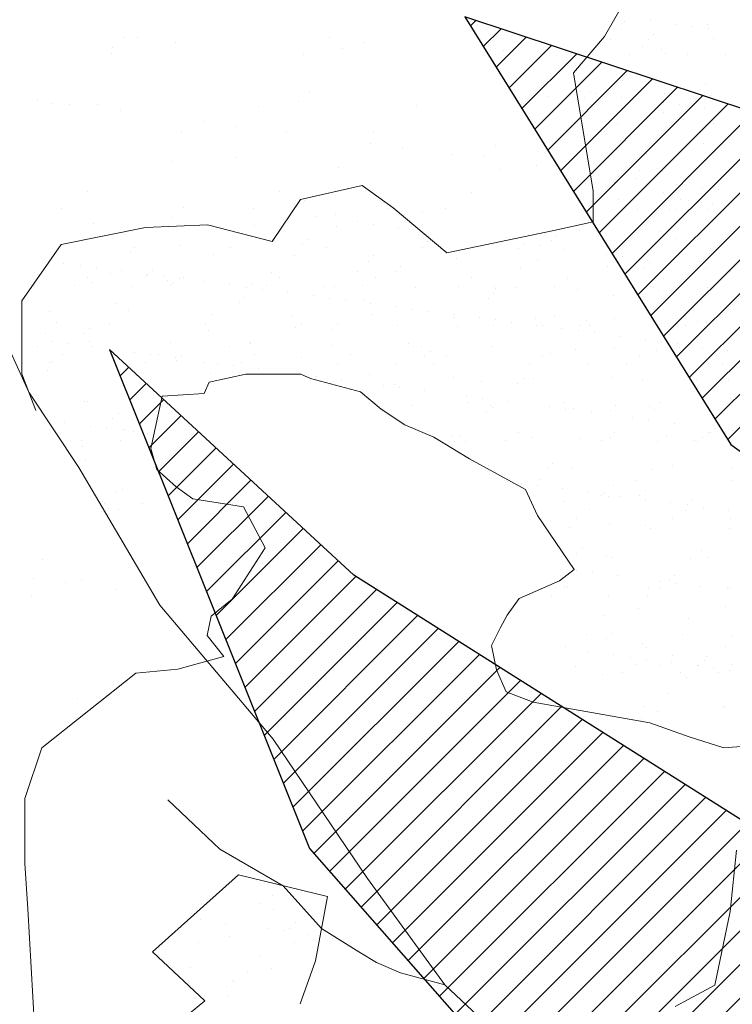
# Model space of a CAD drawing. Units: inches. Extents: x 1986 to 21484, y -1816 to 2016.
# Tile 22 of 85: x 2157.681 to 2162.297, y 1891.95 to 1898.331. Entities that reach past the tile are written whole.
import ezdxf

# ---------------------------------------------------------------- set-up
doc = ezdxf.new("R2010")
doc.units = ezdxf.units.IN
doc.layers.add('L-PLNT', color=84, linetype='Continuous', lineweight=13)
doc.layers.add('vfolhas', color=114, linetype='Continuous', lineweight=5)
doc.layers.add('vfolha2', color=110, linetype='Continuous')
doc.layers.add('vfolhas2', color=102, linetype='Continuous')
pattern_1 = [(45, (-2446.5133113, 50.986076), (-0.004419417382, 0.004419417382), [])]

# ---------------------------------------------------------------- blocks, each defined once
blk = doc.blocks.new('arbusto_PB_verde_grande')
at = {"layer": 'vfolha2'}
h = blk.add_hatch(dxfattribs=at)
h.set_pattern_fill('ANSI31', color=256, scale=0.05, style=0)
h.set_pattern_definition(pattern_1)
h.paths.add_polyline_path([(-0.18963, 0.29704), (-0.08553, 0.20192), (-0.10785, 0.25007), (-0.13202, 0.31865), (-0.25096, 0.48479), (-0.44952, 0.5505), (-0.37946, 0.43789)])
h.paths.add_polyline_path([(0.07911, -0.4071), (0.08214, -0.50631), (0.17255, -0.6355), (0.18428, -0.44151), (0.14904, -0.29177), (0.02625, -0.03934), (0.03527, -0.25376)])
at = {"layer": 'vfolhas'}
h = blk.add_hatch(dxfattribs=at)
h.set_pattern_fill('ANSI31', color=256, scale=0.05, style=0)
h.set_pattern_definition(pattern_1)
h.paths.add_polyline_path([(-0.07279, 0.50669), (-0.18085, 0.65063), (-0.2334, 0.67253), (-0.20712, 0.53176), (-0.10785, 0.25007), (0.02625, -0.03934), (0.00028, 0.09048), (0.00816, 0.16241), (-0.04939, 0.29079)])
h.paths.add_polyline_path([(0.09902, 0.41929), (0.09372, 0.26573), (0.07906, 0.18814), (0.15506, 0.36901), (0.26606, 0.5505), (0.28356, 0.63504), (0.2485, 0.68819), (0.25145, 0.63504), (0.20178, 0.54426)])
h.paths.add_polyline_path([(0.12295, 0.24073), (0.047, 0.06233), (0.02625, -0.03934), (0.11122, 0.04358), (0.18428, 0.09364), (0.27478, 0.19376), (0.3215, 0.25323), (0.44129, 0.38467), (0.47634, 0.57866), (0.41789, 0.45347), (0.28939, 0.30954)])
h.paths.add_polyline_path([(0.58145, -0.03779), (0.70707, 0.01536), (0.78591, 0.04667), (0.74796, 0.06549), (0.62818, 0.08423), (0.52595, 0.09048), (0.39745, 0.04358), (0.02625, -0.03934), (0.25728, -0.03154), (0.43834, -0.0347)])
h.paths.add_polyline_path([(0.52022, -0.03647), (0.43834, -0.0347), (0.25728, -0.03154), (0.02625, -0.03934), (0.17964, -0.08515), (0.53768, -0.13167), (0.69541, -0.15357), (0.78591, -0.07852), (0.70413, -0.10042)])
h.paths.add_polyline_path([(0.27189, -0.21929), (0.14922, -0.14107), (0.02625, -0.03934), (0.15794, -0.31007), (0.29522, -0.42585), (0.41789, -0.49157), (0.56396, -0.56669), (0.5114, -0.48532), (0.39456, -0.34139)])
h.paths.add_polyline_path([(-0.05818, -0.47591), (-0.02312, -0.61984), (0.047, -0.80134), (0.08494, -0.59794), (0.07911, -0.4071), (0.03527, -0.25376), (0.02625, -0.03934), (-0.03773, -0.26001)])
h.paths.add_polyline_path([(-0.24218, 0.14054), (-0.11073, 0.06858), (0.02625, -0.03934), (-0.04235, 0.10871), (-0.21007, 0.23757), (-0.36485, 0.33145), (-0.47874, 0.40341), (-0.54303, 0.46288), (-0.49041, 0.33145), (-0.39408, 0.22192)])
at = {"layer": 'vfolha2'}
for p, q in [((-0.44952, 0.5505), (-0.37946, 0.43789)), ((-0.25096, 0.48479), (-0.44952, 0.5505)), ((-0.37946, 0.43789), (-0.18963, 0.29704))]:
    blk.add_line(p, q, dxfattribs=at)
at = {"layer": 'vfolhas2'}
for p, q in [((-0.54303, 0.46288), (-0.49041, 0.33145)), ((-0.47874, 0.40341), (-0.54303, 0.46288)), ((-0.36485, 0.33145), (-0.47874, 0.40341)), ((-0.49041, 0.33145), (-0.39408, 0.22192))]:
    blk.add_line(p, q, dxfattribs=at)
blk = doc.blocks.new('PLANT-SHRUB')
for p, q in [((2161.4678, 1898.2224), (2161.6137, 1898.4774)), ((2161.5972, 1898.3209), (2161.5972, 1898.3209)), ((2161.7646, 1898.3226), (2161.7646, 1898.3226)), ((2161.9271, 1898.3012), (2161.9271, 1898.3012)), ((2161.9271, 1898.3012), (2161.9271, 1898.3012)), ((2162.0361, 1898.2868), (2162.0361, 1898.2868)), ((2162.1369, 1898.3014), (2162.1369, 1898.3014)), ((2161.2673, 1897.9855), (2161.4678, 1898.2224)), ((2161.5796, 1898.2672), (2161.5796, 1898.2672)), ((2161.5796, 1898.2672), (2161.5796, 1898.2672)), ((2161.7885, 1898.2334), (2161.7885, 1898.2334)), ((2162.1401, 1898.2731), (2162.1401, 1898.2731)), ((2158.3575, 1898.2181), (2158.3575, 1898.2181)), ((2158.4425, 1898.2174), (2158.4425, 1898.2174)), ((2158.6902, 1898.1833), (2158.6902, 1898.1833)), ((2159.6871, 1898.2151), (2159.6871, 1898.2151)), ((2159.9066, 1898.186), (2159.9066, 1898.186)), ((2160.9317, 1898.2128), (2160.9317, 1898.2128)), ((2161.5059, 1898.1997), (2161.5059, 1898.1997)), ((2161.5059, 1898.1997), (2161.5059, 1898.1997)), ((2161.7156, 1898.158), (2161.7156, 1898.158)), ((2161.7517, 1898.1997), (2161.7517, 1898.1997)), ((2162.1764, 1898.2106), (2162.1764, 1898.2106)), ((2162.1764, 1898.2106), (2162.1764, 1898.2106)), ((2158.2739, 1898.11), (2158.2739, 1898.11)), ((2158.2838, 1898.1506), (2158.2838, 1898.1506)), ((2159.5186, 1898.1077), (2159.5186, 1898.1077)), ((2159.7696, 1898.1444), (2159.7696, 1898.1444)), ((2160.7632, 1898.1055), (2160.7632, 1898.1055)), ((2160.8158, 1898.1311), (2160.8158, 1898.1311)), ((2161.6313, 1898.1043), (2161.6313, 1898.1043)), ((2161.8382, 1898.136), (2161.8382, 1898.136)), ((2161.8382, 1898.136), (2161.8382, 1898.136)), ((2161.8667, 1898.1141), (2161.8667, 1898.1141)), ((2162.0078, 1898.1032), (2162.0078, 1898.1032)), ((2162.0078, 1898.1032), (2162.0078, 1898.1032)), ((2162.2536, 1898.1032), (2162.2536, 1898.1032)), ((2161.3949, 1897.2203), (2161.2673, 1897.9855)), ((2161.5528, 1898.0174), (2161.5528, 1898.0174)), ((2161.5846, 1897.9358), (2161.5846, 1897.9358)), ((2162.1244, 1897.9164), (2162.1244, 1897.9164)), ((2159.5589, 1897.8673), (2159.5589, 1897.8673)), ((2161.3139, 1897.8645), (2161.3139, 1897.8645)), ((2161.379, 1897.8581), (2161.379, 1897.8581)), ((2161.4179, 1897.8508), (2161.4179, 1897.8508)), ((2161.8576, 1897.8509), (2161.8576, 1897.8509)), ((2162.1535, 1897.842), (2162.1535, 1897.842)), ((2157.7982, 1897.81), (2157.7982, 1897.81)), ((2157.886, 1897.7861), (2157.886, 1897.7861)), ((2158.0062, 1897.7826), (2158.0062, 1897.7826)), ((2158.183, 1897.783), (2158.183, 1897.783)), ((2159.4853, 1897.7998), (2159.4853, 1897.7998)), ((2161.1081, 1897.8352), (2161.1081, 1897.8352)), ((2161.3421, 1897.8244), (2161.3421, 1897.8244)), ((2161.5804, 1897.8294), (2161.5804, 1897.8294)), ((2161.8518, 1897.7937), (2161.8518, 1897.7937)), ((2161.9558, 1897.78), (2161.9558, 1897.78)), ((2158.3311, 1897.7398), (2158.3311, 1897.7398)), ((2159.2292, 1897.7697), (2159.2292, 1897.7697)), ((2160.2516, 1897.7746), (2160.2516, 1897.7746)), ((2161.3311, 1897.7357), (2161.3311, 1897.7357)), ((2161.3311, 1897.7357), (2161.3311, 1897.7357)), ((2161.3311, 1897.7357), (2161.3311, 1897.7357)), ((2161.8541, 1897.729), (2161.8541, 1897.729)), ((2162.1183, 1897.7586), (2162.1183, 1897.7586)), ((2158.874, 1897.6683), (2158.874, 1897.6683)), ((2161.5542, 1897.6576), (2161.5542, 1897.6576)), ((2161.9429, 1897.649), (2161.9429, 1897.649)), ((2161.9797, 1897.6827), (2161.9797, 1897.6827)), ((2162.1765, 1897.6565), (2162.1765, 1897.6565)), ((2158.7264, 1897.6031), (2158.7264, 1897.6031)), ((2159.082, 1897.6409), (2159.082, 1897.6409)), ((2159.4069, 1897.5982), (2159.4069, 1897.5982)), ((2159.9711, 1897.6008), (2159.9711, 1897.6008)), ((2161.2157, 1897.5986), (2161.2157, 1897.5986)), ((2161.4699, 1897.6039), (2161.4699, 1897.6039)), ((2162.0922, 1897.6028), (2162.0922, 1897.6028)), ((2159.9498, 1897.5267), (2159.9498, 1897.5267)), ((2161.572, 1897.5508), (2161.572, 1897.5508)), ((2162.1118, 1897.5313), (2162.1118, 1897.5313)), ((2160.1578, 1897.4993), (2160.1578, 1897.4993)), ((2160.4828, 1897.4565), (2160.4828, 1897.4565)), ((2160.7604, 1897.5166), (2160.7604, 1897.5166)), ((2161.7439, 1897.4667), (2161.7439, 1897.4667)), ((2158.665, 1897.4132), (2158.665, 1897.4132)), ((2159.0875, 1897.4353), (2159.0875, 1897.4353)), ((2160.6867, 1897.449), (2160.6867, 1897.449)), ((2159.7444, 1897.3743), (2159.7444, 1897.3743)), ((2160.7906, 1897.361), (2160.7906, 1897.361)), ((2161.0256, 1897.3851), (2161.0256, 1897.3851)), ((2161.2337, 1897.3577), (2161.2337, 1897.3577)), ((2161.3961, 1897.3363), (2161.3961, 1897.3363)), ((2161.6962, 1897.3505), (2161.6962, 1897.3505)), ((2161.813, 1897.3659), (2161.813, 1897.3659)), ((2161.813, 1897.3659), (2161.813, 1897.3659)), ((2161.8416, 1897.344), (2161.8416, 1897.344)), ((2161.5333, 1897.2737), (2161.5333, 1897.2737)), ((2161.5586, 1897.3149), (2161.5586, 1897.3149)), ((2161.5586, 1897.3149), (2161.5586, 1897.3149)), ((2161.5701, 1897.3074), (2161.5701, 1897.3074)), ((2161.6676, 1897.3005), (2161.6676, 1897.3005)), ((2161.7716, 1897.2869), (2161.7716, 1897.2869)), ((2161.934, 1897.2655), (2161.934, 1897.2655)), ((2158.1197, 1897.2165), (2158.1197, 1897.2165)), ((2159.3643, 1897.2143), (2159.3643, 1897.2143)), ((2159.4986, 1897.1656), (2159.8997, 1897.2567)), ((2159.8997, 1897.2567), (2160.1003, 1897.1109)), ((2159.8997, 1897.2567), (2159.8997, 1897.2567)), ((2160.6089, 1897.212), (2160.6089, 1897.212)), ((2161.3949, 1897.0199), (2161.3949, 1897.2203)), ((2161.8536, 1897.2098), (2161.8536, 1897.2098)), ((2161.8536, 1897.2098), (2161.8536, 1897.2098)), ((2162.1015, 1897.2434), (2162.1015, 1897.2434)), ((2162.1015, 1897.2434), (2162.1015, 1897.2434)), ((2162.2055, 1897.2297), (2162.2055, 1897.2297)), ((2159.3162, 1896.8923), (2159.4986, 1897.1656)), ((2159.5258, 1897.1606), (2159.5258, 1897.1606)), ((2159.9854, 1897.1894), (2159.9854, 1897.1894)), ((2161.5594, 1897.1657), (2161.5594, 1897.1657)), ((2161.9619, 1897.1658), (2161.9619, 1897.1658)), ((2161.9619, 1897.1658), (2161.9619, 1897.1658)), ((2162.0151, 1897.1561), (2162.0151, 1897.1561)), ((2162.0992, 1897.1463), (2162.0992, 1897.1463)), ((2157.9511, 1897.1092), (2157.9511, 1897.1092)), ((2158.7398, 1897.1167), (2158.7398, 1897.1167)), ((2159.1958, 1897.1069), (2159.1958, 1897.1069)), ((2160.0639, 1897.1058), (2160.0639, 1897.1058)), ((2160.1003, 1897.1109), (2160.4467, 1896.8194)), ((2160.2889, 1897.0845), (2160.2889, 1897.0845)), ((2160.4404, 1897.1046), (2160.4404, 1897.1046)), ((2161.685, 1897.1024), (2161.685, 1897.1024)), ((2161.685, 1897.1024), (2161.685, 1897.1024)), ((2161.8882, 1897.0983), (2161.8882, 1897.0983)), ((2161.8882, 1897.0983), (2161.8882, 1897.0983)), ((2161.9308, 1897.1024), (2161.9308, 1897.1024)), ((2162.134, 1897.0983), (2162.134, 1897.0983)), ((2162.1708, 1897.132), (2162.1708, 1897.132)), ((2157.224, 1897.0515), (2157.739, 1895.9176)), ((2158.1578, 1897.0129), (2158.1578, 1897.0129)), ((2158.6661, 1897.0492), (2158.6661, 1897.0492)), ((2159.5981, 1897.0556), (2159.5981, 1897.0556)), ((2159.7233, 1897.0669), (2159.7233, 1897.0669)), ((2159.8696, 1897.0198), (2159.8696, 1897.0198)), ((2161.1396, 1896.9652), (2161.3949, 1897.0199)), ((2157.9487, 1896.8741), (2158.4957, 1896.9834)), ((2158.4957, 1896.9834), (2158.8968, 1897.0016)), ((2158.4957, 1896.9834), (2158.4957, 1896.9834)), ((2158.8968, 1897.0016), (2159.3162, 1896.8923)), ((2158.8968, 1897.0016), (2158.8968, 1897.0016)), ((2159.204, 1896.9996), (2159.204, 1896.9996)), ((2159.7319, 1896.9893), (2159.7319, 1896.9893)), ((2159.9736, 1897.0062), (2159.9736, 1897.0062)), ((2160.1361, 1896.9848), (2160.1361, 1896.9848)), ((2160.2264, 1897.0045), (2160.2264, 1897.0045)), ((2160.2264, 1897.0045), (2160.2264, 1897.0045)), ((2160.4467, 1896.8194), (2161.1396, 1896.9652)), ((2161.3059, 1896.9656), (2161.3059, 1896.9656)), ((2161.3059, 1896.9656), (2161.3059, 1896.9656)), ((2161.3059, 1896.9656), (2161.3059, 1896.9656)), ((2161.829, 1896.9589), (2161.829, 1896.9589)), ((2159.5495, 1896.9076), (2159.5495, 1896.9076)), ((2160.324, 1896.8915), (2160.324, 1896.8915)), ((2161.1237, 1896.8983), (2161.1237, 1896.8983)), ((2161.1605, 1896.9321), (2161.1605, 1896.9321)), ((2161.9351, 1896.916), (2161.9351, 1896.916)), ((2157.6934, 1896.5097), (2157.9487, 1896.8741)), ((2158.3988, 1896.828), (2158.3988, 1896.828)), ((2158.4232, 1896.8557), (2158.4232, 1896.8557)), ((2158.713, 1896.8669), (2158.713, 1896.8669)), ((2159.0455, 1896.8546), (2159.0455, 1896.8546)), ((2159.5126, 1896.8738), (2159.5126, 1896.8738)), ((2159.6678, 1896.8534), (2159.6678, 1896.8534)), ((2160.2901, 1896.8523), (2160.2901, 1896.8523)), ((2160.4467, 1896.8194), (2160.4467, 1896.8194)), ((2160.9125, 1896.8512), (2160.9125, 1896.8512)), ((2160.9454, 1896.8782), (2160.9454, 1896.8782)), ((2161.0494, 1896.8645), (2161.0494, 1896.8645)), ((2161.2119, 1896.8431), (2161.2119, 1896.8431)), ((2161.5348, 1896.8501), (2161.5348, 1896.8501)), ((2162.1571, 1896.8489), (2162.1571, 1896.8489)), ((2158.9386, 1896.8086), (2158.9386, 1896.8086)), ((2159.4616, 1896.8019), (2159.4616, 1896.8019)), ((2159.9412, 1896.7659), (2159.9412, 1896.7659)), ((2159.9412, 1896.7659), (2159.9412, 1896.7659)), ((2159.9728, 1896.8044), (2159.9728, 1896.8044)), ((2160.5126, 1896.7849), (2160.5126, 1896.7849)), ((2161.0357, 1896.7782), (2161.0357, 1896.7782)), ((2161.4833, 1896.8074), (2161.4833, 1896.8074)), ((2161.5469, 1896.7807), (2161.5469, 1896.7807)), ((2161.5873, 1896.7937), (2161.5873, 1896.7937)), ((2161.7498, 1896.7723), (2161.7498, 1896.7723)), ((2161.7612, 1896.7567), (2161.7612, 1896.7567)), ((2162.0866, 1896.7612), (2162.0866, 1896.7612)), ((2157.9626, 1896.7535), (2157.9626, 1896.7535)), ((2157.9626, 1896.7535), (2157.9626, 1896.7535)), ((2158.0716, 1896.7392), (2158.0716, 1896.7392)), ((2158.1756, 1896.7255), (2158.1756, 1896.7255)), ((2158.3381, 1896.7041), (2158.3381, 1896.7041)), ((2158.5391, 1896.7076), (2158.5391, 1896.7076)), ((2159.3137, 1896.6915), (2159.3137, 1896.6915)), ((2159.8676, 1896.6984), (2159.8676, 1896.6984)), ((2159.8676, 1896.6984), (2159.8676, 1896.6984)), ((2160.1134, 1896.6984), (2160.1134, 1896.6984)), ((2160.1502, 1896.7322), (2160.1502, 1896.7322)), ((2160.9248, 1896.7161), (2160.9248, 1896.7161)), ((2161.4904, 1896.7337), (2161.4904, 1896.7337)), ((2161.4904, 1896.7337), (2161.4904, 1896.7337)), ((2161.7244, 1896.7229), (2161.7244, 1896.7229)), ((2162.0212, 1896.7366), (2162.0212, 1896.7366)), ((2162.1252, 1896.7229), (2162.1252, 1896.7229)), ((2162.2877, 1896.7015), (2162.2877, 1896.7015)), ((2158.1198, 1896.6624), (2158.1198, 1896.6624)), ((2158.1453, 1896.6279), (2158.1453, 1896.6279)), ((2158.2683, 1896.6847), (2158.2683, 1896.6847)), ((2158.2683, 1896.6847), (2158.2683, 1896.6847)), ((2158.5023, 1896.6739), (2158.5023, 1896.6739)), ((2158.5055, 1896.682), (2158.5055, 1896.682)), ((2158.5055, 1896.682), (2158.5055, 1896.682)), ((2158.6095, 1896.6683), (2158.6095, 1896.6683)), ((2158.6398, 1896.6431), (2158.6398, 1896.6431)), ((2158.6398, 1896.6431), (2158.6398, 1896.6431)), ((2158.7135, 1896.6546), (2158.7135, 1896.6546)), ((2158.7135, 1896.6546), (2158.7135, 1896.6546)), ((2158.7135, 1896.6546), (2158.7135, 1896.6546)), ((2158.7421, 1896.6613), (2158.7421, 1896.6613)), ((2158.876, 1896.6333), (2158.876, 1896.6333)), ((2159.3644, 1896.6602), (2159.3644, 1896.6602)), ((2159.9868, 1896.659), (2159.9868, 1896.659)), ((2160.6091, 1896.6579), (2160.6091, 1896.6579)), ((2161.2314, 1896.6568), (2161.2314, 1896.6568)), ((2161.8537, 1896.6557), (2161.8537, 1896.6557)), ((2158.0355, 1896.6088), (2158.0355, 1896.6088)), ((2158.4036, 1896.6023), (2158.4036, 1896.6023)), ((2158.4036, 1896.6023), (2158.4036, 1896.6023)), ((2158.6579, 1896.6076), (2158.6579, 1896.6076)), ((2158.6683, 1896.6212), (2158.6683, 1896.6212)), ((2159.0385, 1896.6119), (2159.0385, 1896.6119)), ((2159.0385, 1896.6119), (2159.0385, 1896.6119)), ((2159.1474, 1896.5975), (2159.1474, 1896.5975)), ((2159.1795, 1896.6237), (2159.1795, 1896.6237)), ((2159.2514, 1896.5838), (2159.2514, 1896.5838)), ((2159.2802, 1896.6065), (2159.2802, 1896.6065)), ((2159.6483, 1896.6), (2159.6483, 1896.6)), ((2159.6483, 1896.6), (2159.6483, 1896.6)), ((2159.7193, 1896.6042), (2159.7193, 1896.6042)), ((2159.7193, 1896.6042), (2159.7193, 1896.6042)), ((2159.7193, 1896.6042), (2159.7193, 1896.6042)), ((2159.9025, 1896.6054), (2159.9025, 1896.6054)), ((2160.2424, 1896.5975), (2160.2424, 1896.5975)), ((2160.5248, 1896.6042), (2160.5248, 1896.6042)), ((2160.7536, 1896.6), (2160.7536, 1896.6)), ((2160.7654, 1896.5909), (2160.7654, 1896.5909)), ((2160.7654, 1896.5909), (2160.7654, 1896.5909)), ((2160.8929, 1896.5977), (2160.8929, 1896.5977)), ((2160.8929, 1896.5977), (2160.8929, 1896.5977)), ((2161.1471, 1896.6031), (2161.1471, 1896.6031)), ((2161.2933, 1896.5805), (2161.2933, 1896.5805)), ((2161.7694, 1896.602), (2161.7694, 1896.602)), ((2161.7878, 1896.5958), (2161.7878, 1896.5958)), ((2161.7878, 1896.5958), (2161.7878, 1896.5958)), ((2161.8164, 1896.5739), (2161.8164, 1896.5739)), ((2162.1375, 1896.5955), (2162.1375, 1896.5955)), ((2162.1375, 1896.5955), (2162.1375, 1896.5955)), ((2157.6934, 1896.036), (2157.6934, 1896.5097)), ((2159.1399, 1896.5322), (2159.1399, 1896.5322)), ((2159.4139, 1896.5624), (2159.4139, 1896.5624)), ((2159.5813, 1896.5404), (2159.5813, 1896.5404)), ((2159.5813, 1896.5404), (2159.5813, 1896.5404)), ((2159.6853, 1896.5267), (2159.6853, 1896.5267)), ((2159.7894, 1896.513), (2159.7894, 1896.513)), ((2159.7894, 1896.513), (2159.7894, 1896.513)), ((2159.7894, 1896.513), (2159.7894, 1896.513)), ((2159.9145, 1896.5162), (2159.9145, 1896.5162)), ((2160.7141, 1896.523), (2160.7141, 1896.523)), ((2160.7509, 1896.5568), (2160.7509, 1896.5568)), ((2161.5255, 1896.5407), (2161.5255, 1896.5407)), ((2157.875, 1896.4405), (2157.875, 1896.4405)), ((2158.3034, 1896.4916), (2158.3034, 1896.4916)), ((2158.3862, 1896.443), (2158.3862, 1896.443)), ((2159.103, 1896.4985), (2159.103, 1896.4985)), ((2159.9518, 1896.4916), (2159.9518, 1896.4916)), ((2160.1143, 1896.4702), (2160.1143, 1896.4702)), ((2160.1143, 1896.4702), (2160.1143, 1896.4702)), ((2160.2232, 1896.4559), (2160.2232, 1896.4559)), ((2160.3273, 1896.4422), (2160.3273, 1896.4422)), ((2158.926, 1896.4235), (2158.926, 1896.4235)), ((2159.4491, 1896.4169), (2159.4491, 1896.4169)), ((2159.9603, 1896.4193), (2159.9603, 1896.4193)), ((2160.4897, 1896.4208), (2160.4897, 1896.4208)), ((2160.5, 1896.3999), (2160.5, 1896.3999)), ((2160.6571, 1896.3988), (2160.6571, 1896.3988)), ((2160.6571, 1896.3988), (2160.6571, 1896.3988)), ((2160.7612, 1896.3851), (2160.7612, 1896.3851)), ((2160.8652, 1896.3714), (2160.8652, 1896.3714)), ((2160.8652, 1896.3714), (2160.8652, 1896.3714)), ((2160.8652, 1896.3714), (2160.8652, 1896.3714)), ((2161.0231, 1896.3932), (2161.0231, 1896.3932)), ((2161.1427, 1896.4151), (2161.1427, 1896.4151)), ((2161.1427, 1896.4151), (2161.1427, 1896.4151)), ((2161.3516, 1896.3814), (2161.3516, 1896.3814)), ((2161.5343, 1896.3956), (2161.5343, 1896.3956)), ((2162.074, 1896.3762), (2162.074, 1896.3762)), ((2157.9206, 1896.3661), (2157.9206, 1896.3661)), ((2157.9206, 1896.3661), (2157.9206, 1896.3661)), ((2158.1295, 1896.3323), (2158.1295, 1896.3323)), ((2158.2618, 1896.3553), (2158.2618, 1896.3553)), ((2158.8841, 1896.3542), (2158.8841, 1896.3542)), ((2158.9041, 1896.3162), (2158.9041, 1896.3162)), ((2159.4698, 1896.3339), (2159.4698, 1896.3339)), ((2159.4698, 1896.3339), (2159.4698, 1896.3339)), ((2159.5064, 1896.353), (2159.5064, 1896.353)), ((2159.7038, 1896.3231), (2159.7038, 1896.3231)), ((2159.7406, 1896.3568), (2159.7406, 1896.3568)), ((2160.1287, 1896.3519), (2160.1287, 1896.3519)), ((2160.5152, 1896.3408), (2160.5152, 1896.3408)), ((2160.7511, 1896.3508), (2160.7511, 1896.3508)), ((2161.0276, 1896.35), (2161.0276, 1896.35)), ((2161.069, 1896.3476), (2161.069, 1896.3476)), ((2161.069, 1896.3476), (2161.069, 1896.3476)), ((2161.1901, 1896.3286), (2161.1901, 1896.3286)), ((2161.1901, 1896.3286), (2161.1901, 1896.3286)), ((2161.2991, 1896.3142), (2161.2991, 1896.3142)), ((2161.3148, 1896.3476), (2161.3148, 1896.3476)), ((2161.3734, 1896.3496), (2161.3734, 1896.3496)), ((2161.9957, 1896.3485), (2161.9957, 1896.3485)), ((2162.1262, 1896.3653), (2162.1262, 1896.3653)), ((2157.8469, 1896.2986), (2157.8469, 1896.2986)), ((2157.8469, 1896.2986), (2157.8469, 1896.2986)), ((2157.8874, 1896.246), (2157.8874, 1896.246)), ((2158.0927, 1896.2986), (2158.0927, 1896.2986)), ((2161.4031, 1896.3006), (2161.4031, 1896.3006)), ((2161.5655, 1896.2792), (2161.5655, 1896.2792)), ((2161.733, 1896.2571), (2161.733, 1896.2571)), ((2161.733, 1896.2571), (2161.733, 1896.2571)), ((2157.7969, 1896.2157), (2157.7969, 1896.2157)), ((2157.7969, 1896.2157), (2157.7969, 1896.2157)), ((2157.9914, 1896.2323), (2157.9914, 1896.2323)), ((2158.1327, 1896.2428), (2158.1327, 1896.2428)), ((2158.1327, 1896.2428), (2158.1327, 1896.2428)), ((2158.1327, 1896.2428), (2158.1327, 1896.2428)), ((2158.1538, 1896.2109), (2158.1538, 1896.2109)), ((2158.6558, 1896.2362), (2158.6558, 1896.2362)), ((2159.0415, 1896.2135), (2159.0415, 1896.2135)), ((2159.0415, 1896.2135), (2159.0415, 1896.2135)), ((2159.1669, 1896.2386), (2159.1669, 1896.2386)), ((2159.1788, 1896.2295), (2159.1788, 1896.2295)), ((2159.1788, 1896.2295), (2159.1788, 1896.2295)), ((2159.7067, 1896.2192), (2159.7067, 1896.2192)), ((2160.2012, 1896.2344), (2160.2012, 1896.2344)), ((2160.2012, 1896.2344), (2160.2012, 1896.2344)), ((2160.2298, 1896.2125), (2160.2298, 1896.2125)), ((2160.2862, 1896.2112), (2160.2862, 1896.2112)), ((2160.2862, 1896.2112), (2160.2862, 1896.2112)), ((2160.3413, 1896.1815), (2160.3413, 1896.1815)), ((2160.741, 1896.2149), (2160.741, 1896.2149)), ((2161.2807, 1896.1955), (2161.2807, 1896.1955)), ((2161.2807, 1896.1955), (2161.2807, 1896.1955)), ((2161.2807, 1896.1955), (2161.2807, 1896.1955)), ((2161.5308, 1896.2089), (2161.5308, 1896.2089)), ((2161.5308, 1896.2089), (2161.5308, 1896.2089)), ((2161.8038, 1896.1888), (2161.8038, 1896.1888)), ((2161.837, 1896.2434), (2161.837, 1896.2434)), ((2161.941, 1896.2297), (2161.941, 1896.2297)), ((2161.941, 1896.2297), (2161.941, 1896.2297)), ((2161.941, 1896.2297), (2161.941, 1896.2297)), ((2161.9524, 1896.206), (2161.9524, 1896.206)), ((2162.1035, 1896.2083), (2162.1035, 1896.2083)), ((2162.2659, 1896.187), (2162.2659, 1896.187)), ((2162.2659, 1896.187), (2162.2659, 1896.187)), ((2157.8938, 1896.1163), (2157.8938, 1896.1163)), ((2157.9584, 1896.162), (2157.9584, 1896.162)), ((2158.4253, 1896.1752), (2158.4253, 1896.1752)), ((2158.5293, 1896.1615), (2158.5293, 1896.1615)), ((2158.5807, 1896.1609), (2158.5807, 1896.1609)), ((2158.6917, 1896.1401), (2158.6917, 1896.1401)), ((2158.6934, 1896.1232), (2158.6934, 1896.1232)), ((2158.7303, 1896.1569), (2158.7303, 1896.1569)), ((2159.2031, 1896.1598), (2159.2031, 1896.1598)), ((2159.5049, 1896.1408), (2159.5049, 1896.1408)), ((2159.8254, 1896.1586), (2159.8254, 1896.1586)), ((2160.3045, 1896.1477), (2160.3045, 1896.1477)), ((2160.4477, 1896.1575), (2160.4477, 1896.1575)), ((2161.07, 1896.1564), (2161.07, 1896.1564)), ((2161.1159, 1896.1654), (2161.1159, 1896.1654)), ((2161.6923, 1896.1552), (2161.6923, 1896.1552)), ((2161.9155, 1896.1722), (2161.9155, 1896.1722)), ((2157.8624, 1896.0555), (2157.8624, 1896.0555)), ((2157.8742, 1896.1083), (2157.8742, 1896.1083)), ((2158.3736, 1896.0579), (2158.3736, 1896.0579)), ((2158.4965, 1896.1072), (2158.4965, 1896.1072)), ((2158.873, 1896.1061), (2158.873, 1896.1061)), ((2158.873, 1896.1061), (2158.873, 1896.1061)), ((2158.9632, 1896.1044), (2158.9632, 1896.1044)), ((2159.0672, 1896.0907), (2159.0672, 1896.0907)), ((2159.1188, 1896.1061), (2159.1188, 1896.1061)), ((2159.2297, 1896.0693), (2159.2297, 1896.0693)), ((2159.7411, 1896.105), (2159.7411, 1896.105)), ((2160.1176, 1896.1038), (2160.1176, 1896.1038)), ((2160.1176, 1896.1038), (2160.1176, 1896.1038)), ((2160.3634, 1896.1038), (2160.3634, 1896.1038)), ((2160.9857, 1896.1027), (2160.9857, 1896.1027)), ((2161.3623, 1896.1016), (2161.3623, 1896.1016)), ((2161.3623, 1896.1016), (2161.3623, 1896.1016)), ((2161.6081, 1896.1016), (2161.6081, 1896.1016)), ((2162.2304, 1896.1004), (2162.2304, 1896.1004)), ((2157.7846, 1895.7991), (2157.6934, 1896.036)), ((2158.9085, 1895.9822), (2159.1461, 1896.0331)), ((2158.9134, 1896.0385), (2158.9134, 1896.0385)), ((2159.1461, 1896.0331), (2159.2706, 1896.0331)), ((2159.2706, 1896.0331), (2159.5025, 1896.0331)), ((2159.5011, 1896.0336), (2159.5011, 1896.0336)), ((2159.5025, 1896.0331), (2159.5647, 1896.0048)), ((2159.5647, 1896.0048), (2159.8872, 1895.92)), ((2159.6051, 1896.0199), (2159.6051, 1896.0199)), ((2159.7676, 1895.9985), (2159.7676, 1895.9985)), ((2159.9477, 1896.0343), (2159.9477, 1896.0343)), ((2160.4874, 1896.0148), (2160.4874, 1896.0148)), ((2160.9421, 1896.0061), (2160.9421, 1896.0061)), ((2161.0105, 1896.0081), (2161.0105, 1896.0081)), ((2161.5217, 1896.0106), (2161.5217, 1896.0106)), ((2161.7166, 1895.99), (2161.7166, 1895.99)), ((2162.0614, 1895.9911), (2162.0614, 1895.9911)), ((2162.2705, 1895.9968), (2162.2705, 1895.9968)), ((2162.2705, 1895.9968), (2162.2705, 1895.9968)), ((2158.4945, 1895.9409), (2158.4945, 1895.9409)), ((2158.8746, 1895.9087), (2158.9085, 1895.9822)), ((2160.039, 1895.9627), (2160.039, 1895.9627)), ((2160.1056, 1895.9654), (2160.1056, 1895.9654)), ((2160.143, 1895.949), (2160.143, 1895.949)), ((2160.3055, 1895.9277), (2160.3055, 1895.9277)), ((2160.6712, 1895.9831), (2160.6712, 1895.9831)), ((2160.6712, 1895.9831), (2160.6712, 1895.9831)), ((2160.9052, 1895.9723), (2160.9052, 1895.9723)), ((2157.739, 1895.9176), (2158.063, 1895.429)), ((2158.5295, 1895.5526), (2158.6031, 1895.8917)), ((2158.6031, 1895.8917), (2158.8746, 1895.9087)), ((2159.8872, 1895.92), (2160.023, 1895.8069)), ((2160.5769, 1895.8919), (2160.5769, 1895.8919)), ((2160.6809, 1895.8782), (2160.6809, 1895.8782)), ((2158.1004, 1895.8549), (2158.1004, 1895.8549)), ((2158.1201, 1895.8578), (2158.1201, 1895.8578)), ((2160.023, 1895.8069), (2160.1757, 1895.7052)), ((2160.2172, 1895.8274), (2160.2172, 1895.8274)), ((2160.5897, 1895.8504), (2160.5897, 1895.8504)), ((2160.7284, 1895.8299), (2160.7284, 1895.8299)), ((2160.7403, 1895.8208), (2160.7403, 1895.8208)), ((2160.7403, 1895.8208), (2160.7403, 1895.8208)), ((2160.8434, 1895.8568), (2160.8434, 1895.8568)), ((2161.1148, 1895.8211), (2161.1148, 1895.8211)), ((2161.212, 1895.8492), (2161.212, 1895.8492)), ((2161.2188, 1895.8074), (2161.2188, 1895.8074)), ((2161.2681, 1895.8105), (2161.2681, 1895.8105)), ((2161.506, 1895.7969), (2161.506, 1895.7969)), ((2161.5428, 1895.8307), (2161.5428, 1895.8307)), ((2161.7627, 1895.8257), (2161.7627, 1895.8257)), ((2161.7627, 1895.8257), (2161.7627, 1895.8257)), ((2161.7912, 1895.8038), (2161.7912, 1895.8038)), ((2161.8343, 1895.8481), (2161.8343, 1895.8481)), ((2158.2839, 1895.7478), (2158.2839, 1895.7478)), ((2158.3207, 1895.7816), (2158.3207, 1895.7816)), ((2160.7063, 1895.7901), (2160.7063, 1895.7901)), ((2161.3813, 1895.786), (2161.3813, 1895.786)), ((2161.6527, 1895.7503), (2161.6527, 1895.7503)), ((2161.7568, 1895.7366), (2161.7568, 1895.7366)), ((2157.9696, 1895.7178), (2157.9696, 1895.7178)), ((2158.137, 1895.6957), (2158.137, 1895.6957)), ((2158.137, 1895.6957), (2158.137, 1895.6957)), ((2158.241, 1895.682), (2158.241, 1895.682)), ((2158.3611, 1895.6729), (2158.3611, 1895.6729)), ((2160.1757, 1895.7052), (2160.3624, 1895.6261)), ((2161.9192, 1895.7152), (2161.9192, 1895.7152)), ((2162.1906, 1895.6795), (2162.1906, 1895.6795)), ((2158.3351, 1895.6068), (2158.3351, 1895.6068)), ((2158.345, 1895.6683), (2158.345, 1895.6683)), ((2158.345, 1895.6683), (2158.345, 1895.6683)), ((2158.345, 1895.6683), (2158.345, 1895.6683)), ((2158.4193, 1895.6605), (2158.4193, 1895.6605)), ((2158.5075, 1895.647), (2158.5075, 1895.647)), ((2160.3235, 1895.6645), (2160.3235, 1895.6645)), ((2160.3235, 1895.6645), (2160.3235, 1895.6645)), ((2160.3624, 1895.6261), (2160.5943, 1895.4848)), ((2160.4748, 1895.6298), (2160.4748, 1895.6298)), ((2160.5325, 1895.6307), (2160.5325, 1895.6307)), ((2160.9086, 1895.656), (2160.9086, 1895.656)), ((2160.9979, 1895.6231), (2160.9979, 1895.6231)), ((2161.3071, 1895.6147), (2161.3071, 1895.6147)), ((2161.5091, 1895.6255), (2161.5091, 1895.6255)), ((2161.5309, 1895.6548), (2161.5309, 1895.6548)), ((2161.8727, 1895.6323), (2161.8727, 1895.6323)), ((2161.8727, 1895.6323), (2161.8727, 1895.6323)), ((2162.0488, 1895.6061), (2162.0488, 1895.6061)), ((2162.1067, 1895.6215), (2162.1067, 1895.6215)), ((2162.1435, 1895.6553), (2162.1435, 1895.6553)), ((2162.1532, 1895.6537), (2162.1532, 1895.6537)), ((2162.2947, 1895.6658), (2162.2947, 1895.6658)), ((2158.0809, 1895.6014), (2158.0809, 1895.6014)), ((2158.0809, 1895.6014), (2158.0809, 1895.6014)), ((2158.085, 1895.5656), (2158.085, 1895.5656)), ((2158.5691, 1895.4169), (2158.5295, 1895.5526)), ((2160.4956, 1895.597), (2160.4956, 1895.597)), ((2160.5701, 1895.5969), (2160.5701, 1895.5969)), ((2160.5701, 1895.5969), (2160.5701, 1895.5969)), ((2160.8243, 1895.6023), (2160.8243, 1895.6023)), ((2161.4467, 1895.6012), (2161.4467, 1895.6012)), ((2161.8148, 1895.5947), (2161.8148, 1895.5947)), ((2161.8148, 1895.5947), (2161.8148, 1895.5947)), ((2162.069, 1895.6), (2162.069, 1895.6)), ((2160.5943, 1895.4848), (2160.9564, 1895.2869)), ((2160.5943, 1895.4848), (2160.5943, 1895.4848)), ((2158.063, 1895.429), (2158.5889, 1894.5368)), ((2158.1075, 1895.4727), (2158.1075, 1895.4727)), ((2158.1075, 1895.4727), (2158.1075, 1895.4727)), ((2158.1075, 1895.4727), (2158.1075, 1895.4727)), ((2158.6936, 1895.3039), (2158.5691, 1895.4169)), ((2160.7158, 1895.4449), (2160.7158, 1895.4449)), ((2161.0964, 1895.4216), (2161.0964, 1895.4216)), ((2161.1332, 1895.4554), (2161.1332, 1895.4554)), ((2161.2555, 1895.4254), (2161.2555, 1895.4254)), ((2161.2555, 1895.4254), (2161.2555, 1895.4254)), ((2161.2555, 1895.4254), (2161.2555, 1895.4254)), ((2161.7786, 1895.4187), (2161.7786, 1895.4187)), ((2161.9078, 1895.4393), (2161.9078, 1895.4393)), ((2162.2898, 1895.4212), (2162.2898, 1895.4212)), ((2158.3485, 1895.2878), (2158.3485, 1895.2878)), ((2158.8011, 1895.2247), (2158.6936, 1895.3039)), ((2160.8216, 1895.3423), (2160.8216, 1895.3423)), ((2160.9306, 1895.328), (2160.9306, 1895.328)), ((2160.9564, 1895.2869), (2161.0356, 1895.1173)), ((2161.0346, 1895.3143), (2161.0346, 1895.3143)), ((2161.0506, 1895.3488), (2161.0506, 1895.3488)), ((2161.1971, 1895.2929), (2161.1971, 1895.2929)), ((2161.525, 1895.3137), (2161.525, 1895.3137)), ((2161.525, 1895.3137), (2161.525, 1895.3137)), ((2161.6729, 1895.3477), (2161.6729, 1895.3477)), ((2162.2952, 1895.3466), (2162.2952, 1895.3466)), ((2158.3029, 1895.2646), (2158.3029, 1895.2646)), ((2158.3029, 1895.2646), (2158.3029, 1895.2646)), ((2159.1292, 1895.1739), (2158.8011, 1895.2247)), ((2160.9853, 1895.238), (2160.9853, 1895.238)), ((2161.3645, 1895.2708), (2161.3645, 1895.2708)), ((2161.3645, 1895.2708), (2161.3645, 1895.2708)), ((2161.4513, 1895.2462), (2161.4513, 1895.2462)), ((2161.4513, 1895.2462), (2161.4513, 1895.2462)), ((2161.4685, 1895.2571), (2161.4685, 1895.2571)), ((2161.4965, 1895.2405), (2161.4965, 1895.2405)), ((2161.5725, 1895.2434), (2161.5725, 1895.2434)), ((2161.5725, 1895.2434), (2161.5725, 1895.2434)), ((2161.5725, 1895.2434), (2161.5725, 1895.2434)), ((2161.6971, 1895.2462), (2161.6971, 1895.2462)), ((2161.7339, 1895.28), (2161.7339, 1895.28)), ((2158.2292, 1895.1971), (2158.2292, 1895.1971)), ((2158.2292, 1895.1971), (2158.2292, 1895.1971)), ((2158.258, 1895.1601), (2158.258, 1895.1601)), ((2158.475, 1895.1971), (2158.475, 1895.1971)), ((2159.1292, 1895.1739), (2159.1292, 1895.1739)), ((2159.2706, 1894.9082), (2159.1292, 1895.1739)), ((2161.208, 1895.2081), (2161.208, 1895.2081)), ((2161.208, 1895.2081), (2161.208, 1895.2081)), ((2161.735, 1895.2221), (2161.735, 1895.2221)), ((2161.8974, 1895.2007), (2161.8974, 1895.2007)), ((2161.8974, 1895.2007), (2161.8974, 1895.2007)), ((2162.0064, 1895.1863), (2162.0064, 1895.1863)), ((2162.0362, 1895.221), (2162.0362, 1895.221)), ((2162.1104, 1895.1726), (2162.1104, 1895.1726)), ((2158.3232, 1895.1538), (2158.3232, 1895.1538)), ((2161.0356, 1895.1173), (2161.2731, 1894.7669)), ((2161.2853, 1895.1007), (2161.2853, 1895.1007)), ((2161.3695, 1895.1544), (2161.3695, 1895.1544)), ((2161.9076, 1895.0996), (2161.9076, 1895.0996)), ((2161.9919, 1895.1533), (2161.9919, 1895.1533)), ((2162.2729, 1895.1512), (2162.2729, 1895.1512)), ((2162.2841, 1895.0985), (2162.2841, 1895.0985)), ((2162.2841, 1895.0985), (2162.2841, 1895.0985)), ((2161.2429, 1895.0404), (2161.2429, 1895.0404)), ((2161.4982, 1895.064), (2161.4982, 1895.064)), ((2161.7375, 1895.0556), (2161.7375, 1895.0556)), ((2161.7375, 1895.0556), (2161.7375, 1895.0556)), ((2161.766, 1895.0337), (2161.766, 1895.0337)), ((2162.2772, 1895.0361), (2162.2772, 1895.0361)), ((2159.0575, 1894.575), (2159.2706, 1894.9082)), ((2161.3243, 1894.9046), (2161.3243, 1894.9046)), ((2161.2875, 1894.8709), (2161.2875, 1894.8709)), ((2161.4839, 1894.8554), (2161.4839, 1894.8554)), ((2161.5115, 1894.8473), (2161.5115, 1894.8473)), ((2162.0989, 1894.8886), (2162.0989, 1894.8886)), ((2162.1338, 1894.8462), (2162.1338, 1894.8462)), ((2157.8314, 1894.8326), (2157.8314, 1894.8326)), ((2162.0237, 1894.836), (2162.0237, 1894.836)), ((2161.2731, 1894.7669), (2161.177, 1894.6934)), ((2161.2842, 1894.764), (2161.2842, 1894.764)), ((2161.3883, 1894.7503), (2161.3883, 1894.7503)), ((2161.5507, 1894.7289), (2161.5507, 1894.7289)), ((2161.9251, 1894.7293), (2161.9251, 1894.7293)), ((2157.7685, 1894.7094), (2157.7685, 1894.7094)), ((2157.9765, 1894.6821), (2157.9765, 1894.6821)), ((2158.0823, 1894.7026), (2158.0823, 1894.7026)), ((2161.177, 1894.6934), (2160.9168, 1894.5803)), ((2161.2081, 1894.654), (2161.2081, 1894.654)), ((2161.2304, 1894.6553), (2161.2304, 1894.6553)), ((2161.2304, 1894.6553), (2161.2304, 1894.6553)), ((2161.2304, 1894.6553), (2161.2304, 1894.6553)), ((2161.7534, 1894.6486), (2161.7534, 1894.6486)), ((2161.8222, 1894.6932), (2161.8222, 1894.6932)), ((2161.8305, 1894.6529), (2161.8305, 1894.6529)), ((2161.8882, 1894.6955), (2161.8882, 1894.6955)), ((2161.9262, 1894.6795), (2161.9262, 1894.6795)), ((2162.0886, 1894.6581), (2162.0886, 1894.6581)), ((2162.2646, 1894.6511), (2162.2646, 1894.6511)), ((2157.7581, 1894.6006), (2157.7581, 1894.6006)), ((2158.3015, 1894.6393), (2158.3015, 1894.6393)), ((2161.1239, 1894.6003), (2161.1239, 1894.6003)), ((2161.492, 1894.5938), (2161.492, 1894.5938)), ((2161.492, 1894.5938), (2161.492, 1894.5938)), ((2161.7462, 1894.5992), (2161.7462, 1894.5992)), ((2162.2765, 1894.642), (2162.2765, 1894.642)), ((2162.2765, 1894.642), (2162.2765, 1894.642)), ((2158.5889, 1894.5368), (2159.3227, 1893.6692)), ((2158.9216, 1894.4663), (2159.0575, 1894.575)), ((2160.9168, 1894.5803), (2160.8376, 1894.4729)), ((2162.255, 1894.5309), (2162.255, 1894.5309)), ((2162.255, 1894.5309), (2162.255, 1894.5309)), ((2158.8944, 1894.3395), (2158.9216, 1894.4663)), ((2160.8376, 1894.4729), (2160.7923, 1894.3882)), ((2161.4713, 1894.4704), (2161.4713, 1894.4704)), ((2161.6893, 1894.5132), (2161.6893, 1894.5132)), ((2162.0111, 1894.451), (2162.0111, 1894.451)), ((2159.0031, 1894.2037), (2158.8944, 1894.3395)), ((2160.7923, 1894.3882), (2160.7357, 1894.2751)), ((2161.3501, 1894.3469), (2161.3501, 1894.3469)), ((2161.5155, 1894.3539), (2161.5155, 1894.3539)), ((2161.9724, 1894.3458), (2161.9724, 1894.3458)), ((2162.2901, 1894.3379), (2162.2901, 1894.3379)), ((2160.7357, 1894.2751), (2160.7697, 1894.1168)), ((2160.7357, 1894.2751), (2160.7357, 1894.2751)), ((2161.2178, 1894.2703), (2161.2178, 1894.2703)), ((2161.4787, 1894.3202), (2161.4787, 1894.3202)), ((2161.7123, 1894.2855), (2161.7123, 1894.2855)), ((2161.7123, 1894.2855), (2161.7123, 1894.2855)), ((2162.252, 1894.266), (2162.252, 1894.266)), ((2158.7041, 1894.1222), (2159.0031, 1894.2037)), ((2161.3665, 1894.2358), (2161.3665, 1894.2358)), ((2161.5289, 1894.2144), (2161.5289, 1894.2144)), ((2161.5289, 1894.2144), (2161.5289, 1894.2144)), ((2161.7408, 1894.2636), (2161.7408, 1894.2636)), ((2161.9073, 1894.2123), (2161.9073, 1894.2123)), ((2161.9073, 1894.2123), (2161.9073, 1894.2123)), ((2162.1299, 1894.205), (2162.1299, 1894.205)), ((2162.1299, 1894.205), (2162.1299, 1894.205)), ((2161.2797, 1894.1379), (2161.2797, 1894.1379)), ((2161.6379, 1894.2), (2161.6379, 1894.2)), ((2161.6691, 1894.1525), (2161.6691, 1894.1525)), ((2161.7419, 1894.1863), (2161.7419, 1894.1863)), ((2161.8336, 1894.1448), (2161.8336, 1894.1448)), ((2161.8336, 1894.1448), (2161.8336, 1894.1448)), ((2161.9044, 1894.1649), (2161.9044, 1894.1649)), ((2162.0718, 1894.1429), (2162.0718, 1894.1429)), ((2162.0718, 1894.1429), (2162.0718, 1894.1429)), ((2162.0794, 1894.1448), (2162.0794, 1894.1448)), ((2162.1162, 1894.1785), (2162.1162, 1894.1785)), ((2162.2914, 1894.1514), (2162.2914, 1894.1514)), ((2157.8249, 1893.6131), (2158.4322, 1894.0951)), ((2158.4322, 1894.0951), (2158.7041, 1894.1222)), ((2160.7697, 1894.1168), (2160.8319, 1893.9755)), ((2161.4587, 1894.0854), (2161.4587, 1894.0854)), ((2161.5848, 1894.0988), (2161.5848, 1894.0988)), ((2161.9613, 1894.0977), (2161.9613, 1894.0977)), ((2161.9613, 1894.0977), (2161.9613, 1894.0977)), ((2162.1758, 1894.1292), (2162.1758, 1894.1292)), ((2162.2071, 1894.0977), (2162.2071, 1894.0977)), ((2162.2798, 1894.1155), (2162.2798, 1894.1155)), ((2162.2798, 1894.1155), (2162.2798, 1894.1155)), ((2162.2798, 1894.1155), (2162.2798, 1894.1155)), ((2161.9985, 1894.0659), (2161.9985, 1894.0659)), ((2160.8319, 1893.9755), (2161.0073, 1893.9077)), ((2161.8805, 1893.9625), (2161.8805, 1893.9625)), ((2158.0571, 1893.9325), (2158.0571, 1893.9325)), ((2161.0073, 1893.9077), (2161.7632, 1893.7743)), ((2161.7283, 1893.8785), (2161.7283, 1893.8785)), ((2161.811, 1893.8453), (2161.811, 1893.8453)), ((2162.2395, 1893.881), (2162.2395, 1893.881)), ((2162.2513, 1893.8719), (2162.2513, 1893.8719)), ((2162.2513, 1893.8719), (2162.2513, 1893.8719)), ((2161.7066, 1893.8032), (2161.7066, 1893.8032)), ((2161.7632, 1893.7743), (2162.0175, 1893.6828)), ((2157.933, 1893.653), (2157.933, 1893.653)), ((2159.3227, 1893.6692), (2159.9342, 1892.7649)), ((2162.0175, 1893.6828), (2162.2413, 1893.6117)), ((2157.7148, 1893.2832), (2157.8249, 1893.6131)), ((2157.8249, 1893.6131), (2157.8249, 1893.6131)), ((2162.2413, 1893.6117), (2162.3532, 1893.6218)), ((2157.7148, 1893.2832), (2157.7148, 1893.2832)), ((2157.7148, 1892.8616), (2157.7148, 1893.2832)), ((2158.6395, 1893.2743), (2158.9777, 1892.9557)), ((2158.9777, 1892.9557), (2159.3871, 1892.7184)), ((2162.3233, 1892.9494), (2162.2835, 1892.5519)), ((2157.7331, 1892.5683), (2157.7148, 1892.8616)), ((2158.5418, 1892.2911), (2159.0987, 1892.788)), ((2159.0987, 1892.788), (2159.6754, 1892.6488)), ((2159.9342, 1892.7649), (2160.4349, 1892.0769)), ((2159.3871, 1892.7184), (2159.6357, 1892.4402)), ((2159.3179, 1892.6547), (2159.3179, 1892.6547)), ((2159.6754, 1892.6488), (2159.5959, 1892.2315)), ((2159.6754, 1892.6488), (2159.6754, 1892.6488)), ((2157.8167, 1891.0729), (2157.7331, 1892.5683)), ((2159.2337, 1892.601), (2159.2337, 1892.601)), ((2159.3232, 1892.5664), (2159.3232, 1892.5664)), ((2162.2835, 1892.5519), (2162.1841, 1892.075)), ((2162.2835, 1892.5519), (2162.2835, 1892.5519)), ((2158.8533, 1892.497), (2158.8533, 1892.497)), ((2159.0157, 1892.4756), (2159.0157, 1892.4756)), ((2159.2872, 1892.4399), (2159.2872, 1892.4399)), ((2159.3912, 1892.4262), (2159.3912, 1892.4262)), ((2159.4307, 1892.4436), (2159.4307, 1892.4436)), ((2159.4675, 1892.4773), (2159.4675, 1892.4773)), ((2159.6357, 1892.4402), (2159.8763, 1892.2895)), ((2159.0411, 1892.3881), (2159.0411, 1892.3881)), ((2159.5537, 1892.4048), (2159.5537, 1892.4048)), ((2159.5808, 1892.3687), (2159.5808, 1892.3687)), ((2158.8799, 1891.9731), (2158.5418, 1892.2911)), ((2158.8376, 1892.3486), (2158.8376, 1892.3486)), ((2159.4599, 1892.3475), (2159.4599, 1892.3475)), ((2159.8763, 1892.2895), (2159.9923, 1892.2219)), ((2159.2318, 1892.2613), (2159.2318, 1892.2613)), ((2159.5959, 1892.2315), (2159.4964, 1891.9533)), ((2157.7504, 1892.2102), (2157.7504, 1892.2102)), ((2158.7875, 1892.188), (2158.7875, 1892.188)), ((2159.3106, 1892.1813), (2159.3106, 1892.1813)), ((2159.9923, 1892.2219), (2160.1469, 1892.1543)), ((2159.0579, 1892.102), (2159.0579, 1892.102)), ((2159.0723, 1892.1006), (2159.0723, 1892.1006)), ((2159.1565, 1892.1542), (2159.1565, 1892.1542)), ((2160.1469, 1892.1543), (2160.4349, 1892.0769)), ((2159.0211, 1892.0683), (2159.0211, 1892.0683)), ((2160.4349, 1892.0769), (2160.8561, 1891.6818)), ((2162.1841, 1892.075), (2161.9255, 1891.9359)), ((2158.1838, 1891.3968), (2158.8799, 1891.9731)), ((2159.0285, 1892.0031), (2159.0285, 1892.0031))]:
    blk.add_line(p, q)

msp = doc.modelspace()

# ---------------------------------------------------------------- block references
at = {"layer": 'L-PLNT'}
msp.add_blockref('PLANT-SHRUB', (0, 0), dxfattribs=at)
at = {"layer": 'L-PLNT', "xscale": 24.60366729364114, "yscale": 24.60366729364114, "zscale": 24.60366729364114}
msp.add_blockref('arbusto_PB_verde_grande', (2171.6234, 1884.8051), dxfattribs=at)

doc.saveas('drawing.dxf')
